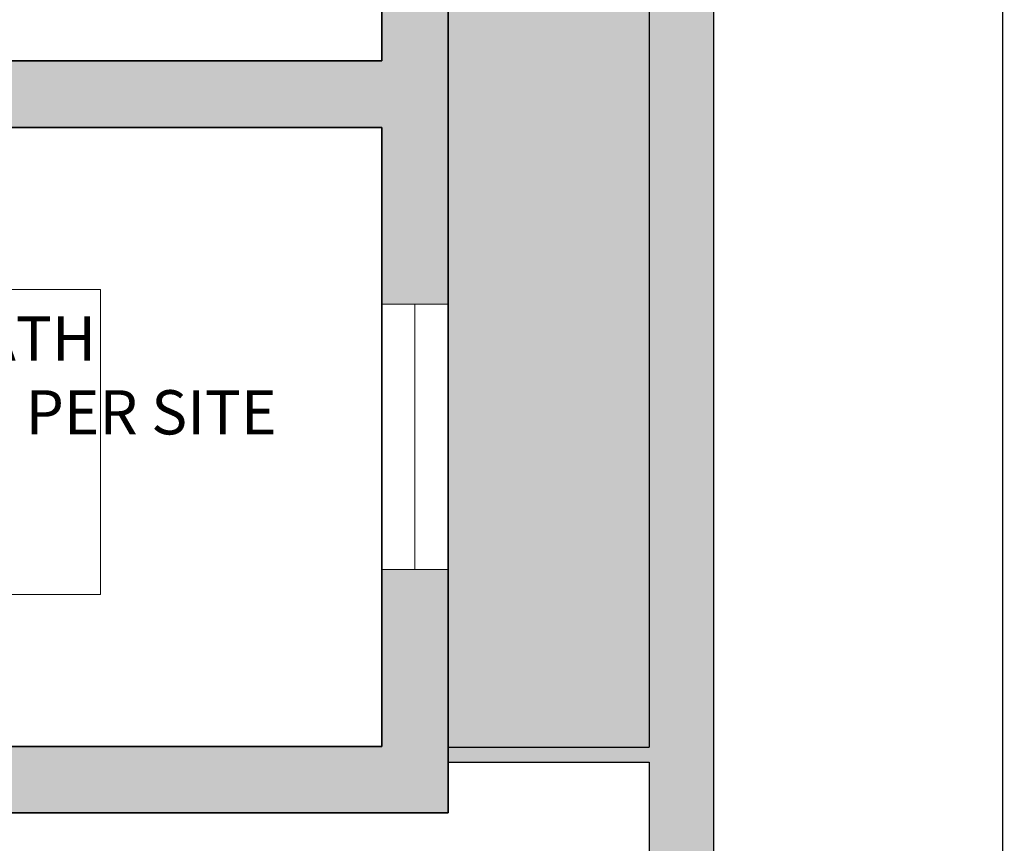
# Model space of a CAD drawing. Units: inches. Extents: x -9 to 646, y -802 to 47.
# Tile 13 of 17: x 512 to 646, y -524 to -412. Entities that reach past the tile are written whole.
import ezdxf

# ---------------------------------------------------------------- set-up
doc = ezdxf.new("R2010")
doc.units = ezdxf.units.IN
doc.header["$MEASUREMENT"] = 0
for name, color, linetype, lineweight in [('A-ANNO-DIMS', 2, 'Continuous', 18), ('A-ANNO-SYMB', 7, 'Continuous', 13), ('A-AREA-IDEN', 7, 'Continuous', 18), ('A-FLOR-PATT', 9, 'Continuous', 9), ('A-GLAZ', 4, 'Continuous', 15), ('A-WALL', 7, 'Continuous', 35), ('A-WALL-PATT', 5, 'Continuous', 9), ('C-SITE', 7, 'Continuous', 25)]:
    doc.layers.add(name, color=color, linetype=linetype, lineweight=lineweight)
doc.styles.get("Standard").update_dxf_attribs({"font": 'arial.ttf'})
doc.dimstyles.get("Standard").update_dxf_attribs({"dimtxt": 0.18, "dimasz": 0.18, "dimexe": 0.18, "dimexo": 0.0625, "dimgap": 0.09, "dimtad": 0, "dimtih": 1, "dimtoh": 1, "dimdec": 0, "dimzin": 0, "dimdsep": 46, "dimlunit": 3, "dimtxsty": 'Standard', "dimcen": 0.09, "dimadec": 0, "dimazin": 0, "dimtfac": 1, "dimtdec": 0, "dimtofl": 0, "dimtmove": 0, "dimatfit": 3, "dimfxl": 1, "dimtolj": 1, "dimtzin": 0, "dimarcsym": 0})

# ---------------------------------------------------------------- blocks, each defined once
blk = doc.blocks.new('GLAZING-36')
for p, q in [((0, 36), (0, 0)), ((4.5, 36), (4.5, 0)), ((9, 0), (9, 36))]:
    blk.add_line(p, q)
blk = doc.blocks.new('*D50')
at = {"layer": 'A-ANNO-DIMS', "color": 0, "lineweight": -2, "transparency": 16777216}
for p, q in [((606.44, 7.93), (645.8, 7.93)), ((645.62, 7.75), (645.62, -376.89)), ((645.62, -761.89), (645.62, -377.25)), ((606.44, -762.07), (645.8, -762.07))]:
    blk.add_line(p, q, dxfattribs=at)
at = {"layer": 'A-ANNO-DIMS', "color": 0, "transparency": 16777216}
for points in [[(645.59, 7.75), (645.65, 7.75), (645.62, 7.93)], [(645.59, -761.89), (645.65, -761.89), (645.62, -762.07)]]:
    blk.add_solid(points, dxfattribs=at)
at = {"layer": 'Defpoints', "color": 0, "transparency": 16777216}
for p in [(606.37, 7.93), (606.37, -762.07), (645.62, -762.07)]:
    blk.add_point(p, dxfattribs=at)
at = {"layer": 'A-ANNO-DIMS', "color": 0, "transparency": 16777216, "insert": (645.62, -377.07), "char_height": 0.18, "attachment_point": 5}
blk.add_mtext('\\A1;770', dxfattribs=at)

msp = doc.modelspace()

# ---------------------------------------------------------------- hatches: boundary and pattern name
at = {"layer": 'A-FLOR-PATT'}
h = msp.add_hatch(dxfattribs=at)
h.set_pattern_fill('AR-HBONE', color=256)
h.paths.add_polyline_path([(597.63, -714.07), (348.37, -714.07), (348.37, -762.07), (597.63, -762.07)])
h.paths.add_polyline_path([(597.63, -101.57), (570.37, -101.57), (570.37, -496.07), (570.37, -511.17), (597.63, -511.17)])
at = {"layer": 'A-WALL-PATT'}
h = msp.add_hatch(color=256, dxfattribs=at)
h.dxf.hatch_style = 1
h.paths.add_polyline_path([(73.4, -418.07), (63.37, -418.07), (63.37, -487.07), (63.35, -496.07), (67.87, -496.07), (67.87, -427.07), (73.4, -427.07)])
h.paths.add_polyline_path([(73.87, -487.07), (67.87, -487.07), (67.87, -496.07), (73.87, -496.07)])
h.paths.add_polyline_path([(39.37, -496.07), (39.35, -496.07), (39.35, -487.07), (30.37, -487.07), (30.37, -646.07), (69.62, -646.07), (69.62, -637.07), (39.37, -637.07)])
h.paths.add_polyline_path([(158.27, -637.07), (105.62, -637.07), (105.62, -646.07), (158.27, -646.07)])
h.paths.add_polyline_path([(286.47, -637.07), (194.27, -637.07), (194.27, -646.07), (286.47, -646.07)])
h.paths.add_polyline_path([(357.37, -552.07), (352.87, -552.07), (348.37, -552.07), (348.37, -637.07), (322.47, -637.07), (322.47, -646.07), (357.37, -646.07)])
h.paths.add_polyline_path([(357.37, -459.07), (352.87, -459.07), (348.37, -459.07), (348.37, -526.07), (357.37, -526.07), (357.37, -520.07), (363.37, -520.07), (363.37, -511.07), (357.37, -511.07)], flags=17)
h.paths.add_polyline_path([(39.37, -262.07), (213.37, -262.07), (213.37, -268.07), (222.37, -268.07), (222.37, -247.07), (213.37, -247.07), (213.37, -253.07), (39.37, -253.07), (39.37, -1.07), (222.37, -1.07), (222.37, 7.93), (30.37, 7.93), (30.37, -427.07), (39.36, -427.07), (39.36, -418.07)])
h.paths.add_polyline_path([(570.37, -149.32), (561.37, -149.32), (561.37, -161.07), (433.37, -161.07), (433.37, -165.57), (433.37, -170.07), (438.37, -170.07), (438.37, -176.07), (447.37, -176.07), (447.37, -170.07), (561.37, -170.07), (561.37, -229.57), (570.37, -229.57)])
h.paths.add_polyline_path([(570.37, -289.57), (561.37, -289.57), (561.37, -349.07), (479.37, -349.07), (479.37, -353.57), (479.37, -358.07), (561.37, -358.07), (561.37, -418.07), (447.37, -418.07), (447.37, -358.07), (453.37, -358.07), (453.37, -349.07), (447.37, -349.07), (447.37, -202.07), (442.87, -202.07), (438.37, -202.07), (438.37, -427.07), (561.37, -427.07), (561.37, -451.07), (570.37, -451.07)])
h.paths.add_polyline_path([(570.37, -496.07), (570.37, -487.07), (561.37, -487.07), (561.37, -511.07), (411.37, -511.07), (411.37, -515.57), (411.37, -520.07), (570.37, -520.07)])
h = msp.add_hatch(color=256, dxfattribs=at)
h.dxf.hatch_style = 1
h.paths.add_polyline_path([(597.63, -101.57), (570.37, -101.57), (570.37, -496.07), (570.37, -511.17), (597.63, -511.17)], flags=0)
h.paths.add_polyline_path([(606.37, -101.57), (597.63, -101.57), (597.63, -511.17), (570.37, -511.17), (570.37, -513.2), (597.63, -513.2), (597.63, -712.07), (606.37, -712.07)])
h = msp.add_hatch(color=256, dxfattribs=at)
h.dxf.hatch_style = 1
h.paths.add_polyline_path([(570.37, -496.07), (570.37, -487.07), (561.37, -487.07), (561.37, -511.07), (411.37, -511.07), (411.37, -515.57), (411.37, -520.07), (570.37, -520.07)])

# ---------------------------------------------------------------- linework, layer by layer
at = {"layer": 'A-ANNO-SYMB'}
for p, q in [((411.37, -449.07), (523.2, -449.07)), ((523.2, -449.07), (523.2, -490.46)), ((523.2, -490.46), (465.37, -490.46))]:
    msp.add_line(p, q, dxfattribs=at)
at = {"layer": 'A-GLAZ'}
for p, q in [((561.37, -451.07), (561.37, -451.07)), ((570.37, -451.07), (561.37, -451.07)), ((561.37, -487.07), (570.37, -487.07))]:
    msp.add_line(p, q, dxfattribs=at)
at = {"layer": 'A-WALL'}
for p, q in [((570.37, -101.57), (570.37, -496.07)), ((561.37, -358.07), (561.37, -418.07)), ((447.37, -418.07), (561.37, -418.07)), ((357.37, -427.07), (561.37, -427.07)), ((561.37, -427.07), (561.37, -511.07)), ((570.37, -496.07), (570.37, -520.07)), ((411.37, -511.07), (561.37, -511.07)), ((411.37, -520.07), (570.37, -520.07))]:
    msp.add_line(p, q, dxfattribs=at)
at = {"layer": 'C-SITE'}
for p, q in [((597.63, -101.57), (597.63, -511.17)), ((606.37, -101.57), (606.37, -762.07)), ((570.37, -511.17), (597.63, -511.17)), ((570.37, -513.2), (597.63, -513.2)), ((597.63, -513.2), (597.63, -762.07))]:
    msp.add_line(p, q, dxfattribs=at)

# ---------------------------------------------------------------- block references
at = {"layer": 'A-GLAZ'}
msp.add_blockref('GLAZING-36', (561.37, -487.07), dxfattribs=at)

# ---------------------------------------------------------------- texts
at = {"layer": 'A-AREA-IDEN', "insert": (501.37, -452.73), "char_height": 6, "attachment_point": 1}
msp.add_mtext('BATH\\PAS PER SITE', dxfattribs=at)

# ---------------------------------------------------------------- dimensions: what is measured, and where the dimension line sits
at = {"layer": 'A-ANNO-DIMS'}
dim = msp.add_linear_dim(base=(645.62, -762.07), p1=(606.37, 7.93), p2=(606.37, -762.07), angle=90, dimstyle='Standard', override={"dimdec": 0, "dimlfac": 1, "dimrnd": 0, "dimzin": 0, "dimdsep": 46, "dimlunit": 2}, dxfattribs=at)
dim.commit()
dim.dimension.update_dxf_attribs({"geometry": '*D50', "text_midpoint": (645.62, -377.07)})

doc.saveas('drawing.dxf')
